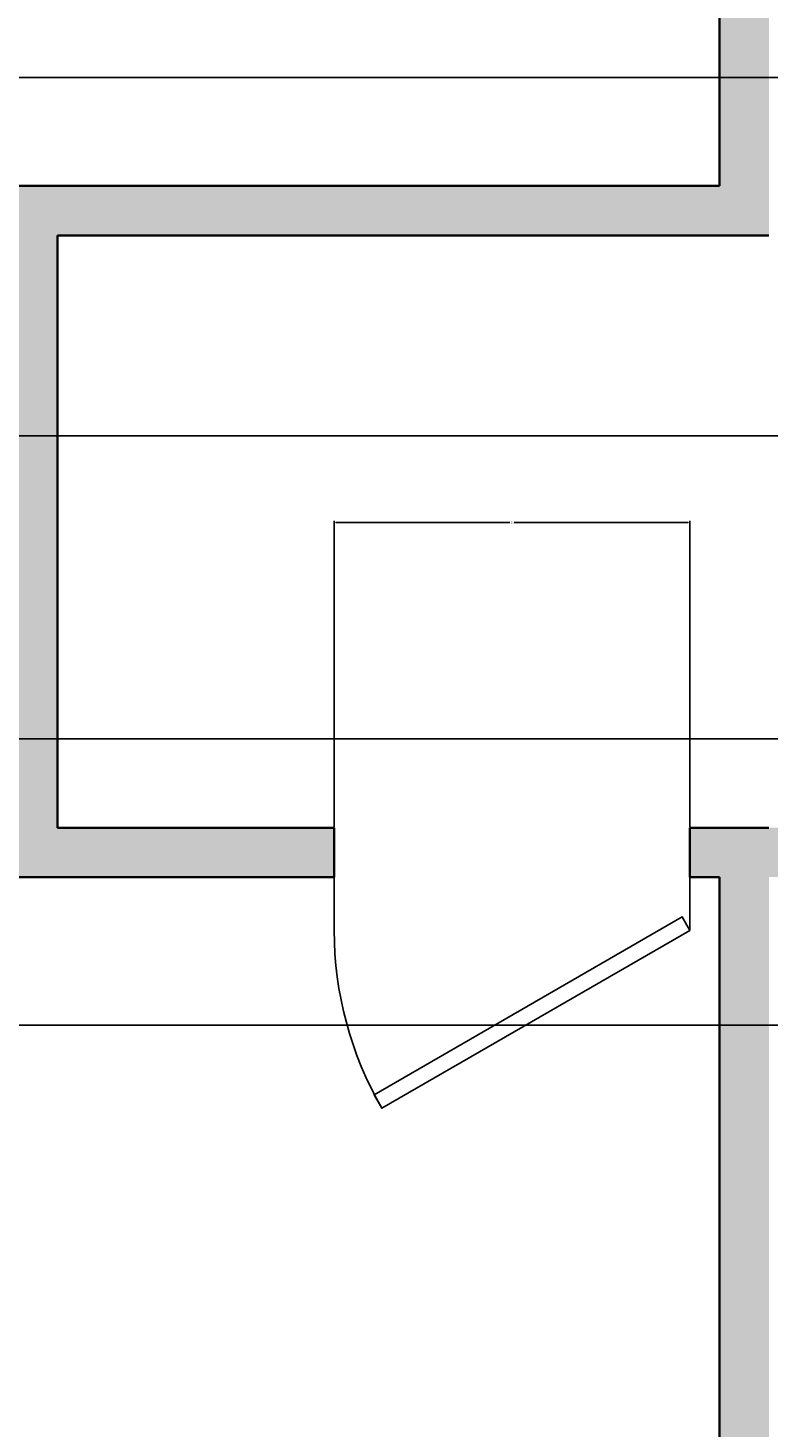
# Model space of a CAD drawing. Units: inches. Extents: x -30 to 437, y -29 to 647.
# Tile 4 of 15: x 97 to 172, y 113 to 255. Entities that reach past the tile are written whole.
import ezdxf

# ---------------------------------------------------------------- set-up
doc = ezdxf.new("R2010")
doc.units = ezdxf.units.IN
doc.header["$MEASUREMENT"] = 0
for name, color, linetype, lineweight in [('A-ANNO-DIMS', 2, 'Continuous', 18), ('A-WALL', 7, 'Continuous', 35), ('doors', 40, 'Continuous', 25)]:
    doc.layers.add(name, color=color, linetype=linetype, lineweight=lineweight)
doc.layers.add('A-WALL-PATT', color=251, linetype='Continuous', lineweight=13, true_color=0x636466)
doc.styles.get("Standard").update_dxf_attribs({"font": 'arial.ttf'})
doc.dimstyles.get("Standard").update_dxf_attribs({"dimtxt": 0.18, "dimasz": 0.18, "dimexe": 0.18, "dimexo": 0.0625, "dimgap": 0.09, "dimtad": 0, "dimtih": 1, "dimtoh": 1, "dimdec": 4, "dimzin": 0, "dimdsep": 46, "dimtxsty": 'Standard', "dimcen": 0.09, "dimadec": 0, "dimazin": 0, "dimtfac": 1, "dimtdec": 4, "dimtofl": 0, "dimtmove": 0, "dimatfit": 3, "dimfxl": 1, "dimtolj": 1, "dimtzin": 0, "dimarcsym": 0})

# ---------------------------------------------------------------- blocks, each defined once
blk = doc.blocks.new('*U6')
for p, q in [((0, 0), (0, -6)), ((40, 0), (40, -6))]:
    blk.add_line(p, q)
blk.add_lwpolyline([(0, 0), (34.64, 20), (35.52, 18.48), (0.87, -1.52)], close=True)
blk.add_arc((0, 0), 40, 0, 30)
blk = doc.blocks.new('*D42')
at = {"layer": 'A-ANNO-DIMS', "color": 0, "lineweight": -2, "transparency": 16777216}
for p, q in [((127.67, 173.61), (127.67, 204.63)), ((127.85, 204.45), (145.45, 204.45)), ((163.49, 204.45), (145.89, 204.45)), ((163.67, 173.61), (163.67, 204.63))]:
    blk.add_line(p, q, dxfattribs=at)
at = {"layer": 'A-ANNO-DIMS', "color": 0, "transparency": 16777216}
for points in [[(127.85, 204.48), (127.85, 204.42), (127.67, 204.45)], [(163.49, 204.48), (163.49, 204.42), (163.67, 204.45)]]:
    blk.add_solid(points, dxfattribs=at)
at = {"layer": 'Defpoints', "color": 0, "transparency": 16777216}
for p in [(163.67, 204.45), (127.67, 173.55), (163.67, 173.55)]:
    blk.add_point(p, dxfattribs=at)
at = {"layer": 'A-ANNO-DIMS', "color": 0, "transparency": 16777216, "insert": (145.67, 204.45), "char_height": 0.18, "attachment_point": 5}
blk.add_mtext('\\A1;36', dxfattribs=at)
blk = doc.blocks.new('*D52')
at = {"layer": 'A-ANNO-DIMS', "color": 0, "lineweight": -2, "transparency": 16777216}
for p, q in [((367.61, 182.55), (-29.41, 182.55)), ((-29.23, 182.37), (-29.23, 168.23)), ((-29.23, 153.73), (-29.23, 167.87)), ((396.61, 153.55), (-29.41, 153.55))]:
    blk.add_line(p, q, dxfattribs=at)
at = {"layer": 'A-ANNO-DIMS', "color": 0, "transparency": 16777216}
for points in [[(-29.26, 182.37), (-29.2, 182.37), (-29.23, 182.55)], [(-29.26, 153.73), (-29.2, 153.73), (-29.23, 153.55)]]:
    blk.add_solid(points, dxfattribs=at)
at = {"layer": 'Defpoints', "color": 0, "transparency": 16777216}
for p in [(367.67, 182.55), (-29.23, 153.55), (396.67, 153.55)]:
    blk.add_point(p, dxfattribs=at)
at = {"layer": 'A-ANNO-DIMS', "color": 0, "transparency": 16777216, "insert": (-29.23, 168.05), "char_height": 0.18, "attachment_point": 5}
blk.add_mtext('\\A1;29', dxfattribs=at)
blk = doc.blocks.new('*D55')
at = {"layer": 'A-ANNO-DIMS', "color": 0, "lineweight": -2, "transparency": 16777216}
for p, q in [((367.61, 249.55), (-29.41, 249.55)), ((-29.23, 249.37), (-29.23, 231.57)), ((-29.23, 213.42), (-29.23, 231.21)), ((369.54, 213.24), (-29.41, 213.24))]:
    blk.add_line(p, q, dxfattribs=at)
at = {"layer": 'A-ANNO-DIMS', "color": 0, "transparency": 16777216}
for points in [[(-29.26, 249.37), (-29.2, 249.37), (-29.23, 249.55)], [(-29.26, 213.42), (-29.2, 213.42), (-29.23, 213.24)]]:
    blk.add_solid(points, dxfattribs=at)
at = {"layer": 'Defpoints', "color": 0, "transparency": 16777216}
for p in [(-29.23, 249.55), (367.67, 249.55), (369.61, 213.24)]:
    blk.add_point(p, dxfattribs=at)
at = {"layer": 'A-ANNO-DIMS', "color": 0, "transparency": 16777216, "insert": (-29.23, 231.39), "char_height": 0.18, "attachment_point": 5}
blk.add_mtext('\\A1;36.31', dxfattribs=at)

msp = doc.modelspace()

# ---------------------------------------------------------------- hatches: boundary and pattern name
at = {"layer": 'A-WALL-PATT'}
h = msp.add_hatch(color=256, dxfattribs=at)
h.dxf.hatch_style = 1
h.paths.add_polyline_path([(393.6054, 183.2352), (369.6054, 183.2352), (369.6054, 213.2352), (393.6054, 213.2352), (393.6054, 207.2352), (394.6054, 207.2352), (394.6054, 211.2352), (395.6054, 211.2352), (395.6054, 185.2352), (394.6054, 185.2352), (394.6054, 189.2352), (393.6054, 189.2352)], flags=0)
h.paths.add_polyline_path([(384.6054, 189.2352, -1), (390.6054, 189.2352, -1)], flags=0)
h.paths.add_polyline_path([(385.6054, 189.2352, -1), (389.6054, 189.2352, -1)], flags=0)
h.paths.add_polyline_path([(374.6054, 189.2352, -1), (382.6054, 189.2352, -1)], flags=0)
h.paths.add_polyline_path([(386.6054, 189.2352, -1), (388.6054, 189.2352, -1)], flags=0)
h.paths.add_polyline_path([(375.6054, 189.2352, -1), (381.6054, 189.2352, -1)], flags=0)
h.paths.add_polyline_path([(376.6054, 189.2352, -1), (380.6054, 189.2352, -1)], flags=0)
h.paths.add_polyline_path([(377.6054, 189.2352, -1), (379.6054, 189.2352, -1)], flags=0)
h.paths.add_polyline_path([(390.6054, 195.2352), (374.6054, 195.2352), (374.6054, 201.2352), (390.6054, 201.2352)], flags=0)
h.paths.add_polyline_path([(389.6054, 196.2352), (375.6054, 196.2352), (375.6054, 200.2352), (389.6054, 200.2352)], flags=0)
h.paths.add_polyline_path([(383.6054, 207.2352, -1), (391.6054, 207.2352, -1)], flags=0)
h.paths.add_polyline_path([(384.6054, 207.2352, -1), (390.6054, 207.2352, -1)], flags=0)
h.paths.add_polyline_path([(385.6054, 207.2352, -1), (389.6054, 207.2352, -1)], flags=0)
h.paths.add_polyline_path([(386.6054, 207.2352, -1), (388.6054, 207.2352, -1)], flags=0)
h.paths.add_polyline_path([(375.6054, 207.2352, -1), (381.6054, 207.2352, -1)], flags=0)
h.paths.add_polyline_path([(376.6054, 207.2352, -1), (380.6054, 207.2352, -1)], flags=0)
h.paths.add_polyline_path([(377.6054, 207.2352, -1), (379.6054, 207.2352, -1)], flags=0)
h.paths.add_polyline_path([(305.5437, 160.3663, -0.41421356), (304.0437, 158.8663), (271.0437, 158.8663, -0.41421356), (269.5437, 160.3663), (269.5437, 178.3663, -0.41421356), (271.0437, 179.8663), (304.0437, 179.8663, -0.41421356), (305.5437, 178.3663)], flags=0)
h.paths.add_polyline_path([(304.0437, 165.3663, -0.41421356), (303.0437, 164.3663), (289.2937, 164.3663, -0.41421356), (288.2937, 165.3663), (288.2937, 177.3663, -0.41421356), (289.2937, 178.3663), (303.0437, 178.3663, -0.41421356), (304.0437, 177.3663)], flags=0)
h.paths.add_polyline_path([(296.5437, 171.3663, -1), (295.5437, 171.3663, -1)], flags=0)
h.paths.add_polyline_path([(286.7937, 165.3663, -0.41421356), (285.7937, 164.3663), (272.0437, 164.3663, -0.41421356), (271.0437, 165.3663), (271.0437, 177.3663, -0.41421356), (272.0437, 178.3663), (285.7937, 178.3663, -0.41421356), (286.7937, 177.3663)], flags=0)
h.paths.add_polyline_path([(279.5437, 171.3663, -1), (278.5437, 171.3663, -1)], flags=0)
h.paths.add_polyline_path([(360.6737, 290.5474), (360.6737, 300.5474), (396.6737, 300.5474), (396.6737, 290.5474)], flags=0)
h.paths.add_polyline_path([(259.6737, 124.5474), (259.6737, 114.5474), (171.6737, 114.5474), (171.6737, 124.5474)], flags=0)
h.paths.add_polyline_path([(288.0737, 215.3705), (286.7097, 214.583), (268.7097, 245.7599), (270.0737, 246.5474)], flags=0)
h.paths.add_polyline_path([(259.6737, 168.5474), (256.6737, 168.5474), (256.6737, 173.5474), (256.6737, 179.0224), (255.8753, 177.6395), (224.2956, 195.872, 0.12053744), (220.1737, 179.0224, 0.12053744), (216.0518, 195.872), (184.4721, 177.6395), (183.6737, 179.0224), (215.2836, 197.2724), (216.0821, 195.8895), (216.0518, 195.872, -0.12053744), (220.1737, 179.0224, -0.12053744), (224.2956, 195.872), (224.2653, 195.8895), (225.0638, 197.2724), (256.6737, 179.0224), (256.6737, 173.5474), (259.6737, 173.5474)], flags=0)
h.paths.add_polyline_path([(386.7943, 325.4601), (372.6871, 325.4601), (372.6871, 339.5673), (386.7943, 339.5673)], flags=0)
h.paths.add_polyline_path([(359.5875, 343.7429), (357.7905, 343.7429), (357.7905, 327.9179), (359.3933, 327.9179, 0.41420885), (361.5302, 330.0549), (361.5302, 341.8434, 0.41436161)], flags=0)
h.paths.add_polyline_path([(341.7887, 323.1235, -0.11921667), (340.7839, 323.1235)], flags=0)
h.paths.add_polyline_path([(379.6332, 328.8632), (379.6332, 332.2699), (376.0992, 332.2699, 0.39427733)], flags=0)
h.paths.add_polyline_path([(375.5299, 332.459, -1), (383.8511, 332.459, -1)], flags=0)
h.paths.add_polyline_path([(388.9363, 344.7425), (372.5309, 344.7425, -0.41421356), (370.394, 346.8794), (370.394, 347.5594, -0.39085173), (372.3472, 349.7005, -0.43951011), (370.394, 351.4933), (370.394, 365.1894, -0.40305452), (372.2191, 367.1298, -0.41839453), (370.394, 368.9291), (370.394, 382.6251, -0.40885826), (372.2519, 384.5722, -0.42377324), (370.394, 386.3707), (370.394, 400.0667, -0.38660687), (372.1327, 402.0094), (372.531, 402.0094, -0.41421834), (370.394, 404.1464), (370.394, 404.7778, -0.41420891), (372.5309, 406.9147), (388.9363, 406.9147, -0.41421821), (391.0733, 404.7778), (391.0733, 346.8794, -0.41421356)], flags=0)
edge = h.paths.add_edge_path(flags=0)
edge.add_spline(control_points=[(349.3585, 363.204), (349.0859, 363.204), (348.8133, 363.2227), (348.2712, 363.2973), (348.0016, 363.3531), (347.3533, 363.5328), (346.9776, 363.6755), (346.2445, 364.0308), (345.887, 364.2432), (345.1953, 364.7329), (344.8611, 365.0101), (344.2197, 365.6237), (343.9125, 365.9603), (343.211, 366.8336), (342.8313, 367.3965), (342.1401, 368.6117), (341.8286, 369.2641), (341.2807, 370.64), (341.0443, 371.3636), (340.6522, 372.8619), (340.4964, 373.6367), (340.2695, 375.2158), (340.1983, 376.0203), (340.142, 377.6365), (340.157, 378.4483), (340.2729, 380.0567), (340.3738, 380.8533), (340.6589, 382.4093), (340.8432, 383.1686), (341.2906, 384.629), (341.5538, 385.3301), (342.1531, 386.6544), (342.4891, 387.2776), (343.2266, 388.4288), (343.6281, 388.9567), (344.4879, 389.9012), (344.9463, 390.3178), (345.7981, 390.9428), (346.182, 391.1771), (346.9712, 391.5648), (347.3766, 391.7182), (348.2004, 391.9387), (348.6189, 392.0058), (349.4588, 392.0508), (349.8801, 392.0288), (350.7146, 391.8966), (351.1278, 391.7865), (351.9366, 391.4822), (352.3323, 391.2882), (353.0989, 390.8223), (353.4699, 390.5504), (354.1819, 389.9355), (354.5229, 389.5924), (355.1706, 388.8418), (355.4772, 388.4343), (356.1315, 387.4422), (356.4671, 386.8397), (357.0692, 385.5581), (357.3356, 384.879), (357.7933, 383.4624), (357.9846, 382.725), (358.2875, 381.2112), (358.3992, 380.4349), (358.5404, 378.8643), (358.5699, 378.0699), (358.546, 376.4841), (358.4926, 375.6928), (358.3042, 374.1343), (358.1692, 373.3672), (357.8207, 371.8774), (357.6072, 371.1549), (357.1067, 369.7735), (356.8196, 369.1148), (356.1782, 367.8787), (355.8238, 367.3013), (355.0551, 366.244), (354.6408, 365.7641), (353.7607, 364.9161), (353.2948, 364.5481), (352.445, 364.0149), (352.0701, 363.822), (351.3034, 363.5117), (350.9116, 363.3943), (350.1325, 363.2418), (349.7455, 363.204), (349.3585, 363.204)], knot_values=[3.14159265, 3.14159265, 3.14159265, 3.14159265, 3.22691715, 3.22691715, 3.31224165, 3.31224165, 3.43426671, 3.43426671, 3.55629177, 3.55629177, 3.67831683, 3.67831683, 3.8003419, 3.8003419, 3.97157384, 3.97157384, 4.14280577, 4.14280577, 4.31403771, 4.31403771, 4.48526965, 4.48526965, 4.65650159, 4.65650159, 4.82773353, 4.82773353, 4.99896547, 4.99896547, 5.1701974, 5.1701974, 5.34142934, 5.34142934, 5.51266128, 5.51266128, 5.68389322, 5.68389322, 5.85512516, 5.85512516, 5.98669107, 5.98669107, 6.11825699, 6.11825699, 6.24982291, 6.24982291, 6.38138882, 6.38138882, 6.51295474, 6.51295474, 6.64452065, 6.64452065, 6.77608657, 6.77608657, 6.90765249, 6.90765249, 7.0392184, 7.0392184, 7.20701563, 7.20701563, 7.37481286, 7.37481286, 7.54261009, 7.54261009, 7.71040732, 7.71040732, 7.87820455, 7.87820455, 8.04600178, 8.04600178, 8.21379901, 8.21379901, 8.38159624, 8.38159624, 8.54939347, 8.54939347, 8.7171907, 8.7171907, 8.88498794, 8.88498794, 9.05278517, 9.05278517, 9.17820699, 9.17820699, 9.30362881, 9.30362881, 9.42477796, 9.42477796, 9.42477796, 9.42477796], degree=3, periodic=0)
edge.add_line((341.1696, 384.3006), (341.2012, 384.2808))
edge = h.paths.add_edge_path(flags=0)
edge.add_line((344.3353, 388.7801), (344.317, 388.7915))
edge.add_ellipse((349.3585, 377.6204), major_axis=(0, -13.7895), ratio=0.62186025, start_angle=-244.867444, end_angle=-124.769923)
h.paths.add_polyline_path([(163.6737, 163.1474), (132.4968, 145.1474), (131.7093, 146.5114), (162.8862, 164.5114)], flags=0)
h.paths.add_polyline_path([(366.4355, 409.0896, -0.41423669), (364.2985, 406.9525, -0.4913499), (361.5302, 408.8973), (361.5302, 420.6405, 0.41421356), (359.3932, 422.7775), (357.7905, 422.7775), (357.7905, 406.9525), (359.6317, 406.9525, 0.42741026), (361.5332, 408.9757, 0.39869469), (363.6672, 406.9525, 0.51958103), (366.4355, 409.0895)], flags=0)
h.paths.add_polyline_path([(386.7943, 410.9671), (372.6871, 410.9671), (372.6871, 425.0742), (386.7943, 425.0742)], flags=0)
h.paths.add_polyline_path([(379.6332, 414.3701), (379.6332, 417.7768), (376.0992, 417.7768, 0.39427733)], flags=0)
h.paths.add_polyline_path([(375.5299, 417.966, -1), (383.8511, 417.966, -1)], flags=0)
h.paths.add_polyline_path([(150.0377, 351.583), (148.6737, 352.3705), (166.6737, 383.5474), (168.0377, 382.7599)], flags=0)
h.paths.add_polyline_path([(91.6737, 234.1974), (66.559, 219.6974), (65.9246, 220.7962), (91.0393, 235.2962)], flags=0)
h.paths.add_polyline_path([(255.4612, 443.5834), (254.6737, 444.9474), (285.8506, 462.9474), (286.6381, 461.5834)], flags=0)
h.paths.add_polyline_path([(176.2737, 394.5474), (158.2737, 425.7243), (159.6377, 426.5118), (177.6377, 395.3349)], flags=0)
h.paths.add_polyline_path([(243.6737, 439.5474), (243.0393, 438.4486), (217.9246, 452.9486), (218.559, 454.0474)], flags=0)
h.paths.add_polyline_path([(38.1264, 269.8429), (40.2408, 269.8429), (40.2408, 270.3508), (38.1264, 270.3508)], flags=0)
h.paths.add_polyline_path([(75.7157, 289.9439), (40.2408, 289.9439), (38.1264, 289.6524), (40.2408, 289.6524)], flags=0)
h.paths.add_polyline_path([(75.7157, 270.0846), (77.6447, 270.0846), (77.6697, 270.1626), (75.7175, 270.1626)], flags=0)
h.paths.add_polyline_path([(80.5373, 293.3002), (33.0467, 293.3002), (13.5054, 293.3002), (13.5054, 351.9244), (29.7898, 351.9244), (80.5373, 351.9244)], flags=0)
h.paths.add_polyline_path([(46.0261, 212.466, -0.50131678), (27.1651, 207.5106), (21.165, 209.5107), (21.165, 206.5107), (22.665, 206.5107), (22.665, 203.5107), (21.165, 203.5107), (21.165, 203.0107), (13.165, 203.0107), (13.165, 224.0107), (21.165, 224.0107), (21.165, 217.5107), (27.1649, 219.5106, -0.50132349), (46.0261, 214.5554, -0.13289091)], flags=0)
h.paths.add_polyline_path([(44.688, 211.8666, -0.48007965), (27.165, 209.5107), (27.165, 217.5107, -0.4800795), (44.688, 215.1547, -0.21500378)], flags=0)
h.paths.add_polyline_path([(19.415, 204.0107), (15.165, 204.0107, -0.41421356), (14.165, 204.7607), (14.165, 222.0107, -0.41421356), (14.915, 223.0107), (19.165, 223.0107, -0.41421356), (20.165, 222.2607), (20.165, 205.0107, -0.41421356)], flags=0)
h.paths.add_polyline_path([(32.7608, 269.0719), (31.8439, 269.0719), (31.8439, 268.6134), (13.5054, 268.6134), (13.5054, 291.5366), (31.8439, 291.5366), (32.7608, 291.0781), (32.7608, 280.9919, -1), (32.7608, 279.1581)], flags=0)
h.paths.add_polyline_path([(40.2408, 360.1436), (38.1264, 360.1436), (38.1264, 359.6357), (40.2408, 359.6357)], flags=0)
h.paths.add_polyline_path([(75.7157, 355.2807), (40.2408, 355.2807), (38.1264, 355.5722), (40.2408, 355.5722), (40.2408, 355.2807), (75.7157, 355.2807), (75.7157, 375.5982), (40.2408, 375.5982), (38.1264, 375.3817), (40.2408, 375.3817), (40.2408, 375.5982), (75.7157, 375.5982), (77.9733, 375.062), (75.7175, 375.062), (75.7175, 374.554)], flags=0)
h.paths.add_polyline_path([(42.8174, 299.814, 0.13867074), (34.1602, 294.603), (14.8081, 294.603), (14.8081, 350.6216), (29.8539, 350.6216, 0.09822056)], flags=0)
h.paths.add_polyline_path([(15.8636, 276.7781, -0.30640166), (20.3757, 283.4499), (20.3483, 290.6726), (31.4014, 290.7146), (31.4309, 282.9124), (26.8287, 282.895, -0.26006276), (30.241, 276.7781, -1)], flags=0)
h.paths.add_polyline_path([(26.1332, 276.7781), (23.0523, 273.6972), (19.9714, 276.7781), (23.0523, 279.8589), (23.0523, 283.9209), (21.3493, 283.9145), (20.7006, 283.5219), (20.6907, 286.1226), (23.2914, 286.1325), (25.8936, 285.7522), (27.1939, 285.7572), (28.4928, 286.1522), (31.0935, 286.1621), (31.0918, 286.6172), (25.6303, 286.5965), (25.616, 290.3675), (31.0775, 290.3882), (31.0918, 286.6172), (31.1034, 283.5614), (28.5027, 283.5515), (25.9005, 283.9317), (23.0523, 283.9209), (23.0523, 279.8589)], flags=0)
h.paths.add_polyline_path([(24.0793, 276.7781, -1), (22.0253, 276.7781, -1)], flags=0)
h.paths.add_polyline_path([(35.7687, 302.2895, -0.41421356), (35.2283, 301.2726), (22.2164, 297.2909, -0.41421356), (21.1995, 297.8313), (15.7317, 315.6996, -0.41421356), (16.2721, 316.7165), (18.8554, 317.507), (15.3721, 328.8904, -0.41421356), (15.9125, 329.9073), (28.9244, 333.889, -0.41421356), (29.9414, 333.3486), (35.4091, 315.4802, -0.41421356), (34.8687, 314.4633), (32.2854, 313.6728)], flags=0)
h.paths.add_polyline_path([(361.3728, 532.6207), (302.7487, 532.6207), (302.7487, 580.1113), (302.7487, 599.6527), (361.3728, 599.6527), (361.3728, 583.3682)], flags=0)
h.paths.add_polyline_path([(370.1, 575.0316), (370.1, 572.9172), (370.6079, 572.9172), (370.6079, 575.0316)], flags=0)
h.paths.add_polyline_path([(385.0466, 537.4423), (385.0466, 572.9172), (384.8302, 575.0316), (384.8302, 572.9172)], flags=0)
h.paths.add_polyline_path([(384.5104, 535.3262), (384.5104, 537.4406), (384.0025, 537.4406), (364.7291, 537.4423), (364.7291, 572.9172), (365.0206, 575.0316), (365.0206, 572.9172), (364.7291, 572.9172), (364.7291, 537.4423), (384.5884, 537.4423), (384.5884, 535.5133)], flags=0)
h.paths.add_polyline_path([(384.5884, 535.5133), (383.4945, 535.164), (383.4945, 537.4406), (382.9866, 535.3262), (382.9866, 537.4406), (383.4945, 535.3262), (383.4945, 537.4406), (384.5884, 537.4406)], flags=0)
h.paths.add_polyline_path([(23.874, 286.8174), (21.0132, 286.8065), (21.0004, 290.1875), (23.8612, 290.1983)], flags=0)
h.paths.add_polyline_path([(242.9824, 511.1667), (234.9824, 511.1667), (234.9824, 517.6667), (228.9825, 515.6667, -0.50132349), (210.1213, 520.622, -0.13289091), (210.1213, 522.7114, -0.50131678), (228.9823, 527.6667), (234.9824, 525.6667), (234.9824, 528.6667), (233.4824, 528.6667), (233.4824, 531.6667), (234.9824, 531.6667), (234.9824, 532.1667), (242.9824, 532.1667)], flags=0)
h.paths.add_polyline_path([(236.9824, 512.1667, -0.41421356), (235.9824, 512.9167), (235.9824, 530.1667, -0.41421356), (236.7324, 531.1667), (240.9824, 531.1667, -0.41421356), (241.9824, 530.4167), (241.9824, 513.1667, -0.41421356), (241.2324, 512.1667)], flags=0)
h.paths.add_polyline_path([(279.533, 537.4423), (279.533, 535.5133), (279.6111, 535.4884), (279.6111, 537.4406)], flags=0)
h.paths.add_polyline_path([(279.2913, 575.0316), (279.2913, 572.9172), (279.7992, 572.9172), (279.7992, 575.0316)], flags=0)
h.paths.add_polyline_path([(211.4594, 520.0227, -0.21500378), (211.4594, 523.3107, -0.48007965), (228.9824, 525.6667), (228.9824, 517.6667, -0.4800795)], flags=0)
h.paths.add_polyline_path([(32.7627, 354.1465), (31.8457, 354.1465), (31.8457, 353.688), (13.5054, 353.688), (13.5054, 376.6134), (31.8457, 376.6134), (32.7627, 376.1549), (32.7627, 366.0677, -1), (32.7627, 364.2337)], flags=0)
h.paths.add_polyline_path([(15.9446, 365.1507, -1), (30.3234, 365.1507, -1)], flags=0)
h.paths.add_polyline_path([(41.213, 428.467), (43.3274, 428.467), (43.3274, 428.9749), (41.213, 428.9749)], flags=0)
h.paths.add_polyline_path([(78.8022, 448.568), (43.3274, 448.568), (41.213, 448.2765), (43.3274, 448.2765)], flags=0)
h.paths.add_polyline_path([(78.8022, 428.7087), (80.7313, 428.7087), (80.7562, 428.7868), (78.804, 428.7868)], flags=0)
h.paths.add_polyline_path([(26.2152, 365.1507), (23.134, 362.0696), (20.0529, 365.1507), (23.134, 368.2319)], flags=0)
h.paths.add_polyline_path([(24.1611, 365.1507, -1), (22.107, 365.1507, -1)], flags=0)
h.paths.add_polyline_path([(309.2625, 570.3406, 0.13867074), (304.0514, 578.9978), (304.0514, 598.3499), (360.07, 598.3499), (360.07, 583.3041, 0.09822056)], flags=0)
h.paths.add_polyline_path([(246.6737, 552.5474), (129.6737, 552.5474), (129.6737, 606.5474), (246.6737, 606.5474)], flags=16)
h.paths.add_polyline_path([(373.6822, 580.3953), (363.595, 580.3953), (363.595, 581.3123), (363.1365, 581.3123), (363.1365, 599.6527), (386.0619, 599.6527), (386.0619, 581.3123), (385.6034, 580.3953), (375.5162, 580.3953, -1)], flags=0)
h.paths.add_polyline_path([(83.6239, 451.9244), (36.1333, 451.9244), (16.5919, 451.9244), (16.5919, 510.5485), (32.8764, 510.5485), (83.6239, 510.5485)], flags=0)
h.paths.add_polyline_path([(367.4098, 590.024, -1), (381.7886, 590.024, -1)], flags=0)
h.paths.add_polyline_path([(374.5992, 586.9428), (371.518, 590.024), (374.5992, 593.1052), (377.6803, 590.024)], flags=0)
h.paths.add_polyline_path([(373.5721, 590.024, -1), (375.6262, 590.024, -1)], flags=0)
h.paths.add_polyline_path([(324.9287, 577.7489, -0.41421356), (323.9118, 578.2893), (323.1212, 580.8726), (311.7379, 577.3893, -0.41421356), (310.721, 577.9297), (306.7393, 590.9416, -0.41421356), (307.2797, 591.9585), (325.1481, 597.4263, -0.41421356), (326.165, 596.8859), (326.9555, 594.3026), (338.3388, 597.7859, -0.41421356), (339.3557, 597.2455), (343.3374, 584.2336, -0.41421356), (342.797, 583.2167)], flags=0)
h.paths.add_polyline_path([(300.5265, 580.3972), (290.4404, 580.3972, -1), (288.6065, 580.3972), (278.5203, 580.3972), (278.5203, 581.3142), (278.0619, 581.3142), (278.0619, 599.6527), (300.985, 599.6527), (300.985, 581.3142)], flags=0)
h.paths.add_polyline_path([(300.163, 581.7567), (292.3609, 581.7271), (292.3434, 586.3294, -0.75567924), (279.0378, 590.1057, -0.82536731), (292.8983, 592.7823), (300.1211, 592.8097)], flags=0)
h.paths.add_polyline_path([(299.8367, 582.0805), (296.0656, 582.0662), (293.0098, 582.0546), (292.9999, 584.6553), (293.3802, 587.2575), (293.3694, 590.1057), (289.3074, 590.1057), (286.2265, 587.0248), (283.1456, 590.1057), (286.2265, 593.1866), (289.3074, 590.1057), (293.3694, 590.1057), (293.3629, 591.8088), (292.9703, 592.4575), (295.5711, 592.4673), (295.5809, 589.8666), (295.2007, 587.2644), (295.2056, 585.9641), (295.6006, 584.6652), (295.6105, 582.0645), (296.0656, 582.0662), (296.0449, 587.5277), (299.8159, 587.542)], flags=0)
h.paths.add_polyline_path([(285.1995, 590.1057, -1), (287.2535, 590.1057, -1)], flags=0)
h.paths.add_polyline_path([(299.6467, 589.2969), (296.2658, 589.284), (296.255, 592.1448), (299.6359, 592.1576)], flags=0)
h.paths.add_polyline_path([(35.8473, 427.696), (34.9304, 427.696), (34.9304, 427.2376), (16.5919, 427.2376), (16.5919, 450.1607), (34.9304, 450.1607), (35.8473, 449.7022), (35.8473, 439.6161, -1), (35.8473, 437.7822)], flags=0)
h.paths.add_polyline_path([(18.9502, 435.4022, -0.30640166), (23.4623, 442.074), (23.4349, 449.2968), (34.4879, 449.3387), (34.5175, 441.5366), (29.9152, 441.5191, -0.26006276), (33.3275, 435.4022, -1)], flags=0)
h.paths.add_polyline_path([(29.2197, 435.4022), (26.1389, 432.3213), (23.058, 435.4022), (26.1389, 438.4831), (26.1389, 442.5451), (24.4358, 442.5386), (23.7871, 442.1461), (23.7772, 444.7468), (26.378, 444.7566), (28.9801, 444.3764), (30.2805, 444.3813), (31.5794, 444.7764), (34.1801, 444.7862), (34.1784, 445.2413), (28.7169, 445.2206), (28.7026, 448.9917), (34.164, 449.0124), (34.1784, 445.2413), (34.1899, 442.1855), (31.5892, 442.1756), (28.987, 442.5559), (26.1389, 442.5451), (26.1389, 438.4831)], flags=0)
h.paths.add_polyline_path([(27.1658, 435.4022, -1), (25.1119, 435.4022, -1)], flags=0)
h.paths.add_polyline_path([(45.904, 458.4382, 0.13867074), (37.2467, 453.2271), (17.8947, 453.2271), (17.8947, 509.2457), (32.9405, 509.2457, 0.09822056)], flags=0)
h.paths.add_polyline_path([(26.9605, 445.4415), (24.0997, 445.4307), (24.0869, 448.8116), (26.9477, 448.8225)], flags=0)
h.paths.add_polyline_path([(38.3149, 459.8967), (25.3029, 455.915, -0.41421356), (24.286, 456.4554), (18.8183, 474.3238, -0.41421356), (19.3586, 475.3407), (21.942, 476.1312), (18.4587, 487.5145, -0.41421356), (18.999, 488.5314), (32.011, 492.5131, -0.41421356), (33.0279, 491.9727), (38.4957, 474.1044, -0.41421356), (37.9553, 473.0875), (35.3719, 472.297), (38.8553, 460.9136, -0.41421356)], flags=0)
h.paths.add_polyline_path([(43.3274, 518.7678), (41.213, 518.7678), (41.213, 518.2598), (43.3274, 518.2598)], flags=0)
h.paths.add_polyline_path([(78.8022, 513.9049), (43.3274, 513.9049), (41.213, 514.1964), (43.3274, 514.1964), (43.3274, 513.9049), (78.8022, 513.9049), (78.8022, 534.2223), (43.3274, 534.2223), (41.213, 534.0059), (43.3274, 534.0059), (43.3274, 534.2223), (78.8022, 534.2223), (81.0599, 533.6861), (78.804, 533.6861), (78.804, 533.1782)], flags=0)
h.paths.add_polyline_path([(121.6737, 556.8974), (121.0393, 555.7986), (95.9246, 570.2986), (96.559, 571.3974)], flags=0)
h.paths.add_polyline_path([(35.8493, 512.7707), (34.9322, 512.7707), (34.9322, 512.3122), (16.5919, 512.3122), (16.5919, 535.2376), (34.9322, 535.2376), (35.8493, 534.7791), (35.8493, 524.6919, -1), (35.8493, 522.8579)], flags=0)
h.paths.add_polyline_path([(19.0312, 523.7749, -1), (33.41, 523.7749, -1)], flags=0)
h.paths.add_polyline_path([(26.2206, 520.6937), (23.1394, 523.7749), (26.2206, 526.8561), (29.3018, 523.7749)], flags=0)
h.paths.add_polyline_path([(25.1935, 523.7749, -1), (27.2476, 523.7749, -1)], flags=0)
h.paths.add_polyline_path([(28.4381, 586.0173), (22.438, 588.0173), (22.438, 585.0173), (23.938, 585.0173), (23.938, 582.0173), (22.438, 582.0173), (22.438, 581.5173), (14.438, 581.5173), (14.438, 602.5173), (22.438, 602.5173), (22.438, 596.0173), (28.4379, 598.0173, -0.50132349), (47.2992, 593.062, -0.13289091), (47.2992, 590.9726, -0.50131678)], flags=0)
h.paths.add_polyline_path([(28.438, 588.0174), (28.438, 596.0173, -0.4800795), (45.961, 593.6614, -0.21500378), (45.961, 590.3733, -0.48007965)], flags=0)
h.paths.add_polyline_path([(20.688, 582.5173), (16.438, 582.5173, -0.41421356), (15.438, 583.2673), (15.438, 600.5173, -0.41421356), (16.188, 601.5173), (20.438, 601.5173, -0.41421356), (21.438, 600.7673), (21.438, 583.5173, -0.41421356)], flags=0)
h.paths.add_polyline_path([(171.6737, 2.0474), (171.6737, 104.5474), (259.6737, 104.5474), (259.6737, 148.5474), (396.6737, 148.5474), (396.6737, 2.0474), (405.6737, 2.0474), (405.6737, 615.5474), (1.6737, 615.5474), (1.6737, 2.0474)])
h.paths.add_polyline_path([(171.6737, 104.5474), (259.6737, 104.5474), (259.6737, 210.5474), (264.6737, 210.5474), (264.6737, 153.5474), (396.6737, 153.5474), (396.6737, 249.5474), (264.6737, 249.5474), (264.6737, 246.5474), (259.6737, 246.5474), (259.6737, 254.5474), (396.6737, 254.5474), (396.6737, 434.5474), (290.6737, 434.5474), (290.6737, 439.5474), (396.6737, 439.5474), (396.6737, 606.5474), (251.6737, 606.5474), (251.6737, 439.5474), (254.6737, 439.5474), (254.6737, 434.5474), (243.6737, 434.5474), (243.6737, 439.5474), (246.6737, 439.5474), (246.6737, 547.5474), (186.6737, 547.5474), (186.6737, 439.5474), (214.6737, 439.5474), (214.6737, 434.5474), (186.6737, 434.5474), (186.6737, 430.5474), (181.6737, 430.5474), (181.6737, 547.5474), (121.6737, 547.5474), (121.6737, 552.5474), (124.6737, 552.5474), (124.6737, 606.5474), (10.6737, 606.5474), (10.6737, 552.5474), (92.6737, 552.5474), (92.6737, 547.5474), (10.6737, 547.5474), (10.6737, 391.5474), (181.6737, 391.5474), (181.6737, 394.5474), (186.6737, 394.5474), (186.6737, 386.5474), (171.6737, 386.5474), (171.6737, 383.5474), (166.6737, 383.5474), (166.6737, 386.5474), (10.6737, 386.5474), (10.6737, 238.5474), (62.6737, 238.5474), (62.6737, 233.5474), (10.6737, 233.5474), (10.6737, 173.5474), (94.6737, 173.5474), (94.6737, 233.5474), (91.6737, 233.5474), (91.6737, 238.5474), (166.6737, 238.5474), (166.6737, 347.5474), (171.6737, 347.5474), (171.6737, 233.5474), (99.6737, 233.5474), (99.6737, 173.5474), (127.6737, 173.5474), (127.6737, 168.5474), (10.6737, 168.5474), (10.6737, 11.0474), (166.6737, 11.0474), (166.6737, 168.5474), (163.6737, 168.5474), (163.6737, 173.5474), (183.6737, 173.5474), (183.6737, 168.5474), (171.6737, 168.5474)])

# ---------------------------------------------------------------- linework, layer by layer
at = {"layer": 'A-WALL'}
for p, q in [((166.6737, 238.5474), (166.6737, 347.5474)), ((91.6737, 238.5474), (166.6737, 238.5474)), ((99.6737, 233.5474), (171.6737, 233.5474)), ((99.6737, 173.5474), (99.6737, 233.5474)), ((99.6737, 173.5474), (127.6737, 173.5474)), ((127.6737, 168.5474), (127.6737, 173.5474)), ((163.6737, 173.5474), (171.6737, 173.5474)), ((166.6737, 173.5474), (163.6737, 173.5474)), ((163.6737, 173.5474), (163.6737, 168.5474)), ((10.6737, 168.5474), (127.6737, 168.5474)), ((163.6737, 168.5474), (166.6737, 168.5474)), ((166.6737, 11.0474), (166.6737, 168.5474))]:
    msp.add_line(p, q, dxfattribs=at)

# ---------------------------------------------------------------- block references
at = {"layer": 'doors', "xscale": 0.9, "yscale": 0.9, "zscale": 0.9, "rotation": 180}
msp.add_blockref('*U6', (163.6737, 163.1474), dxfattribs=at)

# ---------------------------------------------------------------- dimensions: what is measured, and where the dimension line sits
at = {"layer": 'A-ANNO-DIMS'}
for base, p1, p2, override, picture, middle in [((-29.2263, 249.5474), (369.6054, 213.2352), (367.6737, 249.5474), {"dimdec": 2, "dimlfac": 1, "dimrnd": 0, "dimzin": 0, "dimdsep": 46, "dimlunit": 2}, '*D55', (-29.2263, 231.3913)), ((-29.2263, 153.5474), (367.6737, 182.5474), (396.6737, 153.5474), {"dimdec": 0, "dimlfac": 1, "dimrnd": 0, "dimzin": 0, "dimdsep": 46, "dimlunit": 2}, '*D52', (-29.2263, 168.0474))]:
    dim = msp.add_linear_dim(base=base, p1=p1, p2=p2, angle=90, dimstyle='Standard', override=override, dxfattribs=at)
    dim.commit()
    dim.dimension.update_dxf_attribs({"geometry": picture, "text_midpoint": middle})
dim = msp.add_linear_dim(base=(163.6737, 204.4474), p1=(127.6737, 173.5474), p2=(163.6737, 173.5474), dimstyle='Standard', override={"dimdec": 0, "dimlfac": 1, "dimrnd": 0, "dimzin": 0, "dimdsep": 46, "dimlunit": 2}, dxfattribs=at)
dim.commit()
dim.dimension.update_dxf_attribs({"geometry": '*D42', "text_midpoint": (145.6737, 204.4474)})

doc.saveas('drawing.dxf')
